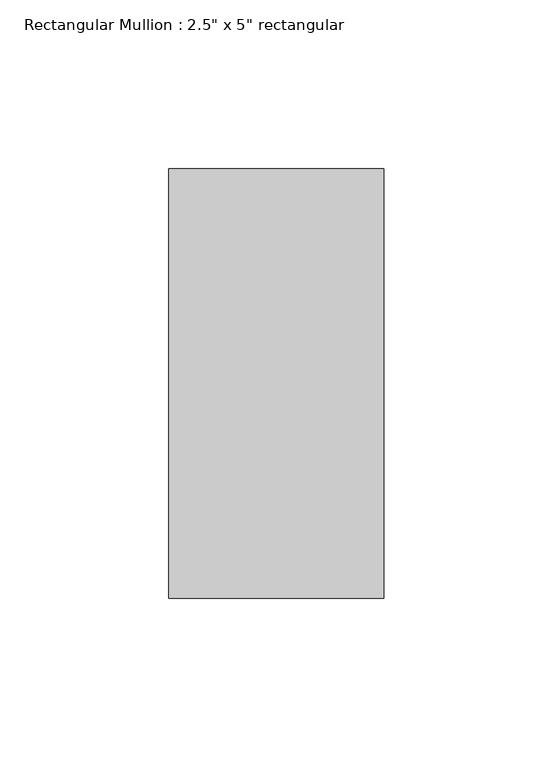
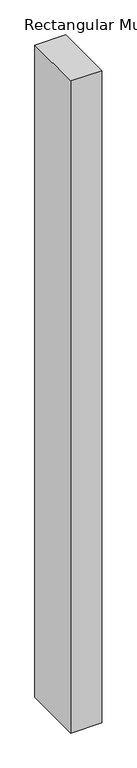
"""IFC4 building model written with IfcOpenShell, lengths in millimetres: member geometry."""

from ifc_helpers import new_model, si_unit, frame, origin, place, context, project, spatial, polyline, outline, extrude, source, transform, mapped, element, save


def member_68d3d74d(model_context):
    return source(origin(), model_context, "Body", "SweptSolid", [
        extrude(outline(polyline([(31.75, 63.5), (31.75, -63.5), (-31.75, -63.5), (-31.75, 63.5), (31.75, 63.5)])), frame((0.0, 0.0, -1409.6999998), z_axis=(0.0, 0.0, 1.0), x_axis=(1.0, 0.0, 0.0)), (0.0, 0.0, 1.0), 1409.6999998),
    ])


if __name__ == "__main__":
    model = new_model("IFC4")
    model_context = context("Model", 3, world=origin())
    ifc_project = project(units=[si_unit("LENGTHUNIT", "METRE", prefix="MILLI")], contexts=[model_context])
    site = spatial("IfcSite", under=ifc_project)
    building = spatial("IfcBuilding", under=site)
    placement = place(None, origin())
    member_shape = member_68d3d74d(model_context)
    element("IfcMember", 1, ObjectType="Rectangular Mullion : 2.5\" x 5\" rectangular", at=placement, inside=building, context=model_context, shape_type="MappedRepresentation", body=[
        mapped(member_shape, transform((0.0, 0.0, 0.0), x_axis=(1.0, 0.0, 0.0), y_axis=(0.0, 1.0, 0.0), z_axis=(0.0, 0.0, 1.0))),
    ])
    save(model, "model.ifc")

# Revit data of these elements
# Type "Rectangular Mullion : 2.5\" x 5\" rectangular"
#   built-in parameter 1007304 = 0.416667 (stored number, unit not read)
#   built-in parameter 1007301 = 0.104167 (stored number, unit not read)
#   built-in parameter 1007300 = 0.104167 (stored number, unit not read)
# Element 1 (IfcMember, "Rectangular Mullion : 2.5\" x 5\" rectangular")
#   Materials on its faces: "WINDOW FRAMING"
# Materials
#   "WINDOW FRAMING": class "Generic", colour RGB 120 120 120, transparency 0, Cost = 0
